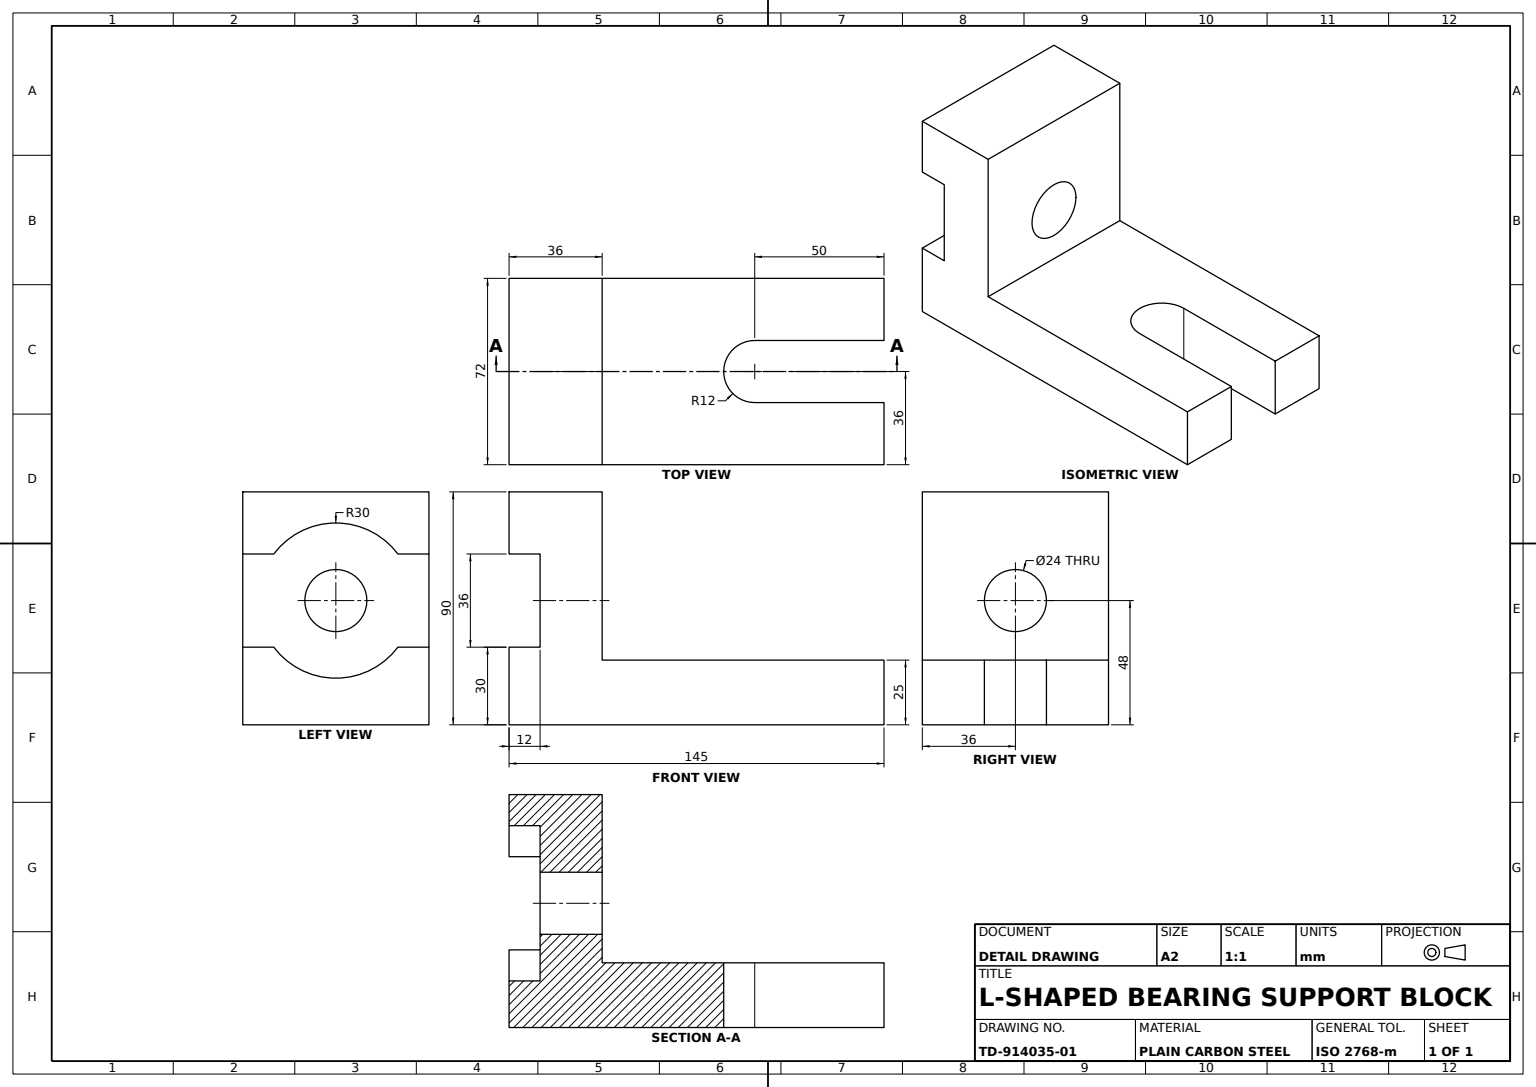
from build123d import *

# Parameters (mm, degrees)
BASE_PLATE_DEPTH       = 25
BASE_SLOT_DEPTH        = 50
UPRIGHT_BLOCK_SKETCH_W = 72
UPRIGHT_BLOCK_SKETCH_H = 36
UPRIGHT_BLOCK_DEPTH    = 65
BEARING_SEAT_CUT_DEPTH = 12
THROUGH_BORE_SKETCH_R  = 12
THROUGH_BORE_DEPTH     = 106


with BuildPart() as part:
    # Base Plate Sketch → Base Plate (new body)
    with BuildSketch(Plane(origin=(0, 0, 0), x_dir=(1, 0, 0), z_dir=(0, 1, 0))):
        Polygon((36, 0), (36, 72.5), (-36, 72.5), (-36, -72.5), (36, -72.5), align=None)
    extrude(amount=BASE_PLATE_DEPTH)

    # Base Slot Sketch → Base Slot (cut)
    with BuildSketch(Plane(origin=(0, 25, 0), x_dir=(1, 0, 0), z_dir=(0, 1, 0))):
        with BuildLine():
            Line((12, 22.5), (12, 72.5))
            Line((12, 72.5), (-12, 72.5))
            Line((-12, 72.5), (-12, 22.5))
            ThreePointArc((-12, 22.5), (0, 10.5), (12, 22.5))
        make_face()
    extrude(amount=-BASE_SLOT_DEPTH, mode=Mode.SUBTRACT)

    # Upright Block Sketch → Upright Block (add)
    with BuildSketch(Plane(origin=(0, 25, 0), x_dir=(1, 0, 0), z_dir=(0, 1, 0))):
        with Locations((0, -54.5)):
            Rectangle(UPRIGHT_BLOCK_SKETCH_W, UPRIGHT_BLOCK_SKETCH_H)
    extrude(amount=UPRIGHT_BLOCK_DEPTH)

    # Bearing Seat Sketch → Bearing Seat Cut (cut)
    with BuildSketch(Plane.XY.offset(72.5)):
        with BuildLine():
            Line((-36, 66), (-36, 30))
            Line((-36, 30), (-24, 30))
            ThreePointArc((-24, 30), (0, 18), (24, 30))
            Line((24, 30), (36, 30))
            Line((36, 30), (36, 66))
            Line((36, 66), (24, 66))
            ThreePointArc((24, 66), (0, 78), (-24, 66))
            Line((-24, 66), (-36, 66))
        make_face()
    extrude(amount=-BEARING_SEAT_CUT_DEPTH, mode=Mode.SUBTRACT)

    # Through Bore Sketch → Through Bore (cut)
    with BuildSketch(Plane.XY.offset(60.5)):
        with Locations((0, 48)):
            Circle(THROUGH_BORE_SKETCH_R)
    extrude(amount=-THROUGH_BORE_DEPTH, mode=Mode.SUBTRACT)


solid = part.part
